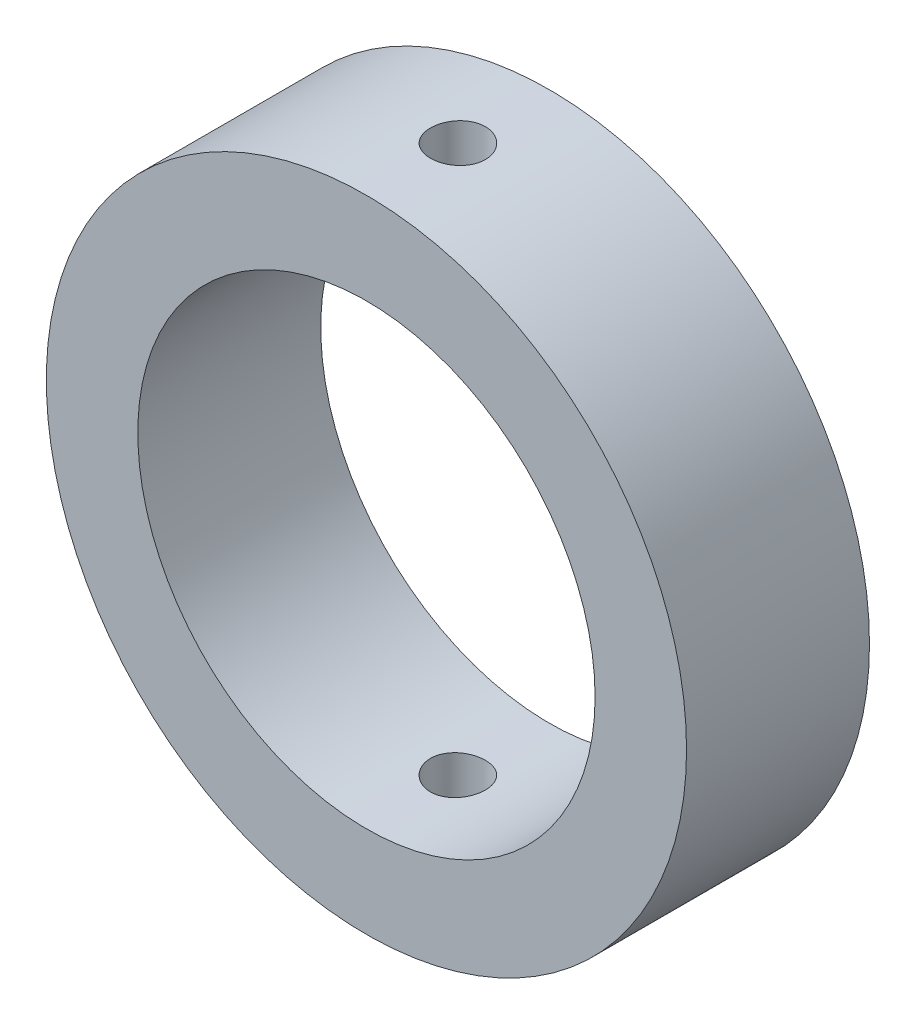
from build123d import *

# Parameters (mm, degrees)
COLLAR_RING_SKETCH_70_50_R   = 35
COLLAR_RING_SKETCH_70_50_R_2 = 25
COLLAR_RING_20_THICK_DEPTH   = 20
RADIAL_PIN_HOLE_6_DEPTH      = 54.38539126
RADIAL_PIN_HOLE_6_DEPTH_BACK = 54.38539126
PIN_HOLE_SKETCH_6_R          = 3


with BuildPart() as part:
    # Collar Ring Sketch Ø70-Ø50 → Collar Ring 20 Thick (new body)
    with BuildSketch(Plane.XY):
        Circle(COLLAR_RING_SKETCH_70_50_R)
        Circle(COLLAR_RING_SKETCH_70_50_R_2, mode=Mode.SUBTRACT)
    extrude(amount=COLLAR_RING_20_THICK_DEPTH)

    # Pin Hole Sketch Ø6 → Radial Pin Hole Ø6 (cut, two sides: drawn at the far end of the back side and taken through both)
    with BuildSketch(Plane(origin=(0, 0, 0), x_dir=(1, 0, 0), z_dir=(0, 1, 0)).offset(-RADIAL_PIN_HOLE_6_DEPTH_BACK)):
        with Locations(Location((0, -10, 0), (0, 0, 270))):
            Circle(PIN_HOLE_SKETCH_6_R)
    extrude(amount=RADIAL_PIN_HOLE_6_DEPTH + RADIAL_PIN_HOLE_6_DEPTH_BACK, mode=Mode.SUBTRACT)


solid = part.part
